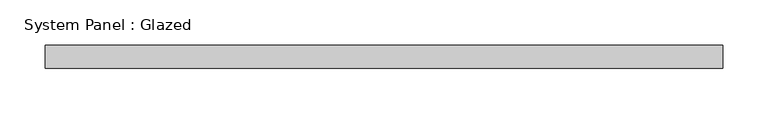
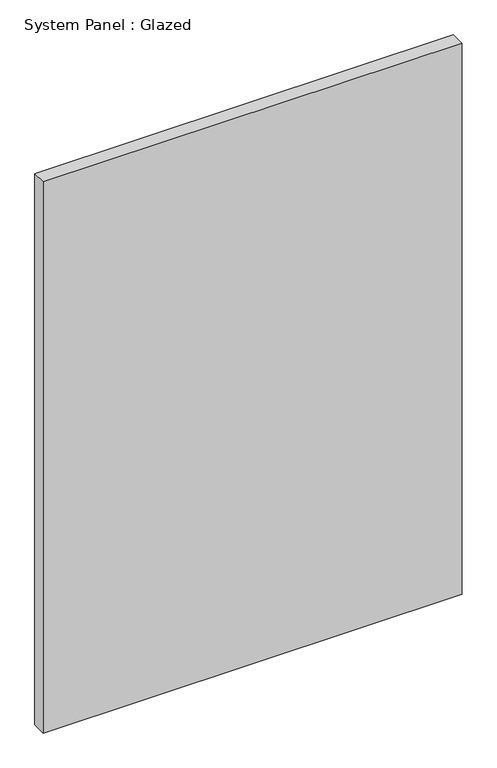
"""IFC4 building model written with IfcOpenShell, lengths in millimetres: plate geometry, System Panel : Glazed."""

from ifc_helpers import new_model, si_unit, origin, origin_with_axes, place, context, project, spatial, polyline, outline, extrude, source, transform, mapped, element, save


def system_panel_glazed_ceb8c9d8(model_context):
    return source(origin(), model_context, "Body", "SweptSolid", [
        extrude(outline(polyline([(374.65, 19.05), (-374.65, 19.05), (-374.65, 44.45), (374.65, 44.45), (374.65, 19.05)])), origin_with_axes(), (0.0, 0.0, 1.0), 1042.1148635),
    ])


if __name__ == "__main__":
    model = new_model("IFC4")
    model_context = context("Model", 3, world=origin())
    ifc_project = project(units=[si_unit("LENGTHUNIT", "METRE", prefix="MILLI")], contexts=[model_context])
    site = spatial("IfcSite", under=ifc_project)
    building = spatial("IfcBuilding", under=site)
    placement = place(None, origin())
    system_panel_glazed_shape = system_panel_glazed_ceb8c9d8(model_context)
    element("IfcPlate", 1, ObjectType="System Panel : Glazed", at=placement, inside=building, context=model_context, shape_type="MappedRepresentation", body=[
        mapped(system_panel_glazed_shape, transform((0.0, 0.0, 0.0), x_axis=(1.0, 0.0, 0.0), y_axis=(0.0, 1.0, 0.0), z_axis=(0.0, 0.0, 1.0))),
    ])
    save(model, "model.ifc")

# Revit data of these elements
# Type "System Panel : Glazed"
#   Construction Type Id = "GSP4R"
#   Analytic Construction = "1/8 in Pilkington single glazing"
#   Visual Light Transmittance = 0.9
#   Solar Heat Gain Coefficient = 0.86
#   Heat Transfer Coefficient (U) = 1.18115 BTU/(h·ft²·°F)
#   Define Thermal Properties by = 1
# Element 1 (IfcPlate, "System Panel : Glazed")
#   Materials on its faces: "Glass"
# Materials
#   "Glass": class "Glass", colour RGB 0 128 192, transparency 0.75, Description = "Soda Lime Glass", Cost = 0
